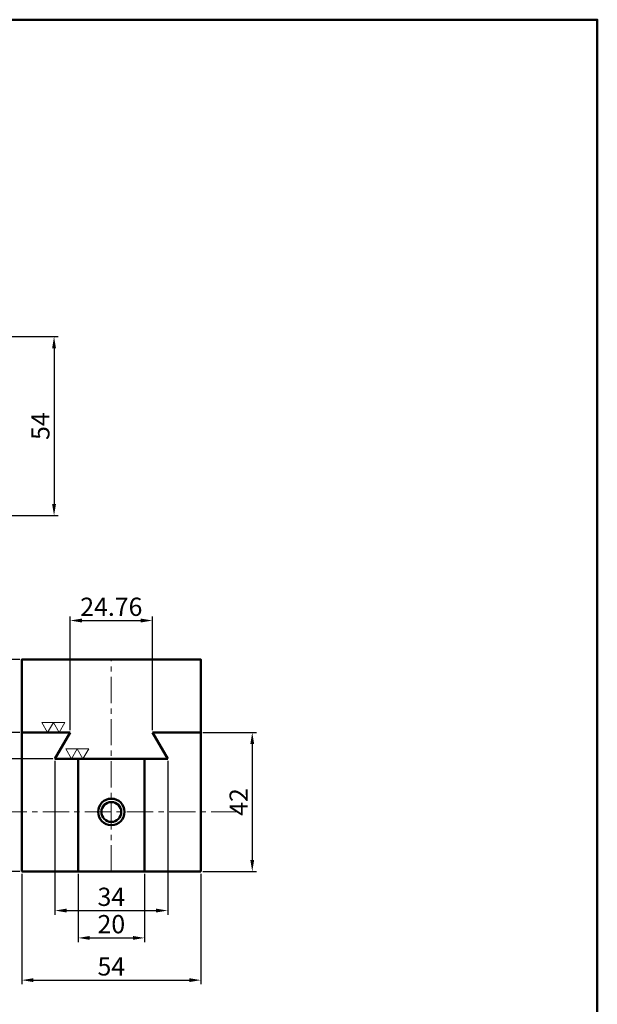
# Model space of a CAD drawing. Units: millimetres. Extents: x 10 to 613, y -226 to 271.
# Tile 4 of 4: x 439 to 613, y -26 to 271. Entities that reach past the tile are written whole.
import ezdxf

# ---------------------------------------------------------------- set-up
doc = ezdxf.new("R2010")
doc.units = ezdxf.units.MM
doc.header["$LTSCALE"] = 0.5
doc.linetypes.add('CENTER', pattern=[50.8, 31.75, -6.35, 6.35, -6.35])
for name, color, linetype, lineweight in [('M-CNTR', 1, 'CENTER', 18), ('M-DIMS', 2, 'Continuous', 25), ('M-OUTL', 7, 'Continuous', 50), ('M-SYMB', 2, 'Continuous', 18), ('M-TTLB', 7, 'Continuous', 50)]:
    doc.layers.add(name, color=color, linetype=linetype, lineweight=lineweight)
doc.styles.get("Standard").update_dxf_attribs({"font": 'arial.ttf'})
doc.dimstyles.new('ISO-25', dxfattribs={"dimtxt": 5.5, "dimasz": 3.5, "dimexe": 1.25, "dimexo": 0.625, "dimtad": 1, "dimtoh": 1, "dimtxsty": 'Standard', "dimcen": 2.5, "dimadec": 0, "dimazin": 0, "dimtfac": 1, "dimtmove": 0, "dimatfit": 3, "dimfxl": 1, "dimarcsym": 0})

# ---------------------------------------------------------------- blocks, each defined once
blk = doc.blocks.new('*D35')
at = {"layer": 'Defpoints', "color": 0, "ltscale": 0.5, "transparency": 16777216}
for p in [(439.79, 77.64), (434.32, 13.64), (439.79, 13.64)]:
    blk.add_point(p, dxfattribs=at)
at = {"layer": 'M-DIMS', "color": 0, "lineweight": -2, "ltscale": 0.5, "transparency": 16777216}
for p, q in [((439.17, 77.64), (433.07, 77.64)), ((434.32, 74.14), (434.32, 17.14)), ((439.17, 13.64), (433.07, 13.64))]:
    blk.add_line(p, q, dxfattribs=at)
at = {"layer": 'M-DIMS', "color": 0, "ltscale": 0.5, "transparency": 16777216}
for points in [[(433.74, 74.14), (434.9, 74.14), (434.32, 77.64)], [(433.74, 17.14), (434.9, 17.14), (434.32, 13.64)]]:
    blk.add_solid(points, dxfattribs=at)
at = {"layer": 'M-DIMS', "color": 0, "ltscale": 0.5, "transparency": 16777216, "insert": (430.89, 45.64), "char_height": 5.5, "attachment_point": 5, "rotation": 90}
blk.add_mtext('64', dxfattribs=at)
blk = doc.blocks.new('*D36')
at = {"layer": 'Defpoints', "color": 0, "ltscale": 0.5, "transparency": 16777216}
for p in [(493.79, 55.64), (493.79, 13.64), (509.31, 13.64)]:
    blk.add_point(p, dxfattribs=at)
at = {"layer": 'M-DIMS', "color": 0, "lineweight": -2, "ltscale": 0.5, "transparency": 16777216}
for p, q in [((494.42, 55.64), (510.56, 55.64)), ((509.31, 52.14), (509.31, 17.14)), ((494.42, 13.64), (510.56, 13.64))]:
    blk.add_line(p, q, dxfattribs=at)
at = {"layer": 'M-DIMS', "color": 0, "ltscale": 0.5, "transparency": 16777216}
for points in [[(508.73, 52.14), (509.89, 52.14), (509.31, 55.64)], [(508.73, 17.14), (509.89, 17.14), (509.31, 13.64)]]:
    blk.add_solid(points, dxfattribs=at)
at = {"layer": 'M-DIMS', "color": 0, "ltscale": 0.5, "transparency": 16777216, "insert": (505.92, 34.64), "char_height": 5.5, "attachment_point": 5, "rotation": 90}
blk.add_mtext('42', dxfattribs=at)
blk = doc.blocks.new('*D37')
at = {"layer": 'Defpoints', "color": 0, "ltscale": 0.5, "transparency": 16777216}
for p in [(456.79, 13.64), (476.79, 13.64), (476.79, -6.36)]:
    blk.add_point(p, dxfattribs=at)
at = {"layer": 'M-DIMS', "color": 0, "lineweight": -2, "ltscale": 0.5, "transparency": 16777216}
for p, q in [((456.79, 13.02), (456.79, -7.61)), ((476.79, 13.02), (476.79, -7.61)), ((460.29, -6.36), (473.29, -6.36))]:
    blk.add_line(p, q, dxfattribs=at)
at = {"layer": 'M-DIMS', "color": 0, "ltscale": 0.5, "transparency": 16777216}
for points in [[(460.29, -5.77), (460.29, -6.94), (456.79, -6.36)], [(473.29, -5.77), (473.29, -6.94), (476.79, -6.36)]]:
    blk.add_solid(points, dxfattribs=at)
at = {"layer": 'M-DIMS', "color": 0, "ltscale": 0.5, "transparency": 16777216, "insert": (466.79, -2.92), "char_height": 5.5, "attachment_point": 5}
blk.add_mtext('20', dxfattribs=at)
blk = doc.blocks.new('*D38')
at = {"layer": 'Defpoints', "color": 0, "ltscale": 0.5, "transparency": 16777216}
for p in [(439.79, 13.64), (493.79, 13.64), (493.79, -19.09)]:
    blk.add_point(p, dxfattribs=at)
at = {"layer": 'M-DIMS', "color": 0, "lineweight": -2, "ltscale": 0.5, "transparency": 16777216}
for p, q in [((439.79, 13.02), (439.79, -20.34)), ((493.79, 13.02), (493.79, -20.34)), ((443.29, -19.09), (490.29, -19.09))]:
    blk.add_line(p, q, dxfattribs=at)
at = {"layer": 'M-DIMS', "color": 0, "ltscale": 0.5, "transparency": 16777216}
for points in [[(443.29, -18.51), (443.29, -19.68), (439.79, -19.09)], [(490.29, -18.51), (490.29, -19.68), (493.79, -19.09)]]:
    blk.add_solid(points, dxfattribs=at)
at = {"layer": 'M-DIMS', "color": 0, "ltscale": 0.5, "transparency": 16777216, "insert": (466.79, -15.67), "char_height": 5.5, "attachment_point": 5}
blk.add_mtext('54', dxfattribs=at)
blk = doc.blocks.new('*D45')
at = {"layer": 'Defpoints', "color": 0, "ltscale": 0.5, "transparency": 16777216}
for p in [(414.06, 175.04), (414.06, 121.04), (449.51, 121.04)]:
    blk.add_point(p, dxfattribs=at)
at = {"layer": 'M-DIMS', "color": 0, "lineweight": -2, "ltscale": 0.5, "transparency": 16777216}
for p, q in [((414.68, 175.04), (450.76, 175.04)), ((449.51, 171.54), (449.51, 124.54)), ((414.68, 121.04), (450.76, 121.04))]:
    blk.add_line(p, q, dxfattribs=at)
at = {"layer": 'M-DIMS', "color": 0, "ltscale": 0.5, "transparency": 16777216}
for points in [[(448.93, 171.54), (450.09, 171.54), (449.51, 175.04)], [(448.93, 124.54), (450.09, 124.54), (449.51, 121.04)]]:
    blk.add_solid(points, dxfattribs=at)
at = {"layer": 'M-DIMS', "color": 0, "ltscale": 0.5, "transparency": 16777216, "insert": (446.09, 148.04), "char_height": 5.5, "attachment_point": 5, "rotation": 90}
blk.add_mtext('54', dxfattribs=at)
blk = doc.blocks.new('SYM-SURF-FINISH-B')
at = {"ltscale": 0.5}
for points in [[(445.84, 58.64), (447.57, 55.64), (449.3, 58.64)], [(449.3, 58.64), (451.03, 55.64), (452.76, 58.64)]]:
    blk.add_lwpolyline(points, close=True, dxfattribs=at)
blk = doc.blocks.new('*D59')
at = {"layer": 'Defpoints', "color": 0, "ltscale": 0.5, "transparency": 16777216}
for p in [(479.17, 89.39), (454.41, 55.64), (479.17, 55.64)]:
    blk.add_point(p, dxfattribs=at)
at = {"layer": 'M-DIMS', "color": 0, "lineweight": -2, "ltscale": 0.5, "transparency": 16777216}
for p, q in [((454.41, 56.27), (454.41, 90.64)), ((457.91, 89.39), (475.67, 89.39)), ((479.17, 56.27), (479.17, 90.64))]:
    blk.add_line(p, q, dxfattribs=at)
at = {"layer": 'M-DIMS', "color": 0, "ltscale": 0.5, "transparency": 16777216}
for points in [[(457.91, 89.98), (457.91, 88.81), (454.41, 89.39)], [(475.67, 89.98), (475.67, 88.81), (479.17, 89.39)]]:
    blk.add_solid(points, dxfattribs=at)
at = {"layer": 'M-DIMS', "color": 0, "ltscale": 0.5, "transparency": 16777216, "insert": (466.79, 92.83), "char_height": 5.5, "attachment_point": 5}
blk.add_mtext('24.76', dxfattribs=at)
blk = doc.blocks.new('*D60')
at = {"layer": 'Defpoints', "color": 0, "ltscale": 0.5, "transparency": 16777216}
for p in [(449.79, 47.64), (483.79, 47.64), (483.79, 1.89)]:
    blk.add_point(p, dxfattribs=at)
at = {"layer": 'M-DIMS', "color": 0, "lineweight": -2, "ltscale": 0.5, "transparency": 16777216}
for p, q in [((449.79, 47.02), (449.79, 0.64)), ((483.79, 47.02), (483.79, 0.64)), ((453.29, 1.89), (480.29, 1.89))]:
    blk.add_line(p, q, dxfattribs=at)
at = {"layer": 'M-DIMS', "color": 0, "ltscale": 0.5, "transparency": 16777216}
for points in [[(453.29, 2.48), (453.29, 1.31), (449.79, 1.89)], [(480.29, 2.48), (480.29, 1.31), (483.79, 1.89)]]:
    blk.add_solid(points, dxfattribs=at)
at = {"layer": 'M-DIMS', "color": 0, "ltscale": 0.5, "transparency": 16777216, "insert": (466.79, 5.33), "char_height": 5.5, "attachment_point": 5}
blk.add_mtext('34', dxfattribs=at)
blk = doc.blocks.new('*D61')
at = {"layer": 'Defpoints', "color": 0, "ltscale": 0.5, "transparency": 16777216}
for p in [(439.79, 55.64), (282.33, 47.64), (449.79, 47.64)]:
    blk.add_point(p, dxfattribs=at)
at = {"layer": 'M-DIMS', "color": 0, "lineweight": -2, "ltscale": 0.5, "transparency": 16777216}
for p, q in [((282.33, 59.14), (282.33, 62.64)), ((439.17, 55.64), (281.08, 55.64)), ((282.33, 55.64), (282.33, 47.64)), ((449.17, 47.64), (281.08, 47.64)), ((282.33, 44.14), (282.33, 40.64))]:
    blk.add_line(p, q, dxfattribs=at)
at = {"layer": 'M-DIMS', "color": 0, "ltscale": 0.5, "transparency": 16777216}
for points in [[(281.75, 59.14), (282.92, 59.14), (282.33, 55.64)], [(281.75, 44.14), (282.92, 44.14), (282.33, 47.64)]]:
    blk.add_solid(points, dxfattribs=at)
at = {"layer": 'M-DIMS', "color": 0, "ltscale": 0.5, "transparency": 16777216, "insert": (278.9, 51.64), "char_height": 5.5, "attachment_point": 5, "rotation": 90}
blk.add_mtext('8', dxfattribs=at)

msp = doc.modelspace()

# ---------------------------------------------------------------- linework, layer by layer
at = {"layer": 'M-CNTR', "ltscale": 0.5}
for p, q in [((466.79, 13.642), (466.79, 77.642)), ((504.837, 31.642), (430.858, 31.642))]:
    msp.add_line(p, q, dxfattribs=at)
at = {"layer": 'M-OUTL', "ltscale": 0.5}
for p, q in [((439.79, 55.642), (454.409, 55.642)), ((445.79, 55.642), (454.409, 55.642)), ((449.79, 47.642), (454.409, 55.642)), ((479.172, 55.642), (487.79, 55.642)), ((483.79, 47.642), (479.172, 55.642)), ((479.172, 55.642), (493.79, 55.642)), ((449.79, 47.642), (483.79, 47.642)), ((456.79, 13.642), (456.79, 47.642)), ((476.79, 13.642), (476.79, 47.642)), ((439.79, 13.642), (493.79, 13.642))]:
    msp.add_line(p, q, dxfattribs=at)
msp.add_lwpolyline([(439.79, 13.642), (439.79, 77.642), (493.79, 77.642), (493.79, 76.642), (493.79, 13.642)], dxfattribs=at)
for radius in [4, 3]:
    msp.add_circle((466.79, 31.642), radius, dxfattribs=at)
at = {"layer": 'M-TTLB', "ltscale": 0.5}
msp.add_lwpolyline([(9.692, 270.659), (613.416, 270.659), (613.416, -225.522), (9.692, -225.522)], close=True, dxfattribs=at)

# ---------------------------------------------------------------- block references
at = {"layer": 'M-SYMB'}
for p in [(0, 0), (7.2, -8)]:
    msp.add_blockref('SYM-SURF-FINISH-B', p, dxfattribs=at)

# ---------------------------------------------------------------- dimensions: what is measured, and where the dimension line sits
at = {"layer": 'M-DIMS', "ltscale": 0.5}
for base, p1, p2, override, picture, middle in [((449.511, 121.041), (414.058, 175.041), (414.058, 121.041), {"dimclrd": 0, "dimclre": 0, "dimclrt": 0}, '*D45', (446.089, 148.041)), ((434.32, 13.642), (439.79, 77.642), (439.79, 13.642), {"dimclrd": 0, "dimclre": 0, "dimclrt": 0}, '*D35', (430.887, 45.642)), ((282.334, 47.642), (439.79, 55.642), (449.79, 47.642), {"dimdec": 0, "dimlfac": 1, "dimrnd": 0, "dimzin": 0, "dimdsep": 46, "dimlunit": 2}, '*D61', (278.901, 51.642)), ((509.309, 13.642), (493.79, 55.642), (493.79, 13.642), {"dimclrd": 0, "dimclre": 0, "dimclrt": 0}, '*D36', (505.923, 34.642))]:
    dim = msp.add_linear_dim(base=base, p1=p1, p2=p2, angle=90, dimstyle='ISO-25', override=override, dxfattribs=at)
    dim.commit()
    dim.dimension.update_dxf_attribs({"geometry": picture, "text_midpoint": middle})
for base, p1, p2, override, picture, middle in [((479.172, 89.392), (454.409, 55.642), (479.172, 55.642), {"dimdec": 2, "dimlfac": 1, "dimrnd": 0, "dimzin": 0, "dimdsep": 46, "dimlunit": 2}, '*D59', (466.79, 92.825)), ((483.79, 1.892), (449.79, 47.642), (483.79, 47.642), {"dimdec": 0, "dimlfac": 1, "dimrnd": 0, "dimzin": 0, "dimdsep": 46, "dimlunit": 2}, '*D60', (466.79, 5.327)), ((493.79, -19.094), (439.79, 13.642), (493.79, 13.642), {"dimclrd": 0, "dimclre": 0, "dimclrt": 0}, '*D38', (466.79, -15.672)), ((476.79, -6.357), (456.79, 13.642), (476.79, 13.642), {"dimclrd": 0, "dimclre": 0, "dimclrt": 0}, '*D37', (466.79, -2.924))]:
    dim = msp.add_linear_dim(base=base, p1=p1, p2=p2, dimstyle='ISO-25', override=override, dxfattribs=at)
    dim.commit()
    dim.dimension.update_dxf_attribs({"geometry": picture, "text_midpoint": middle})

doc.saveas('drawing.dxf')
